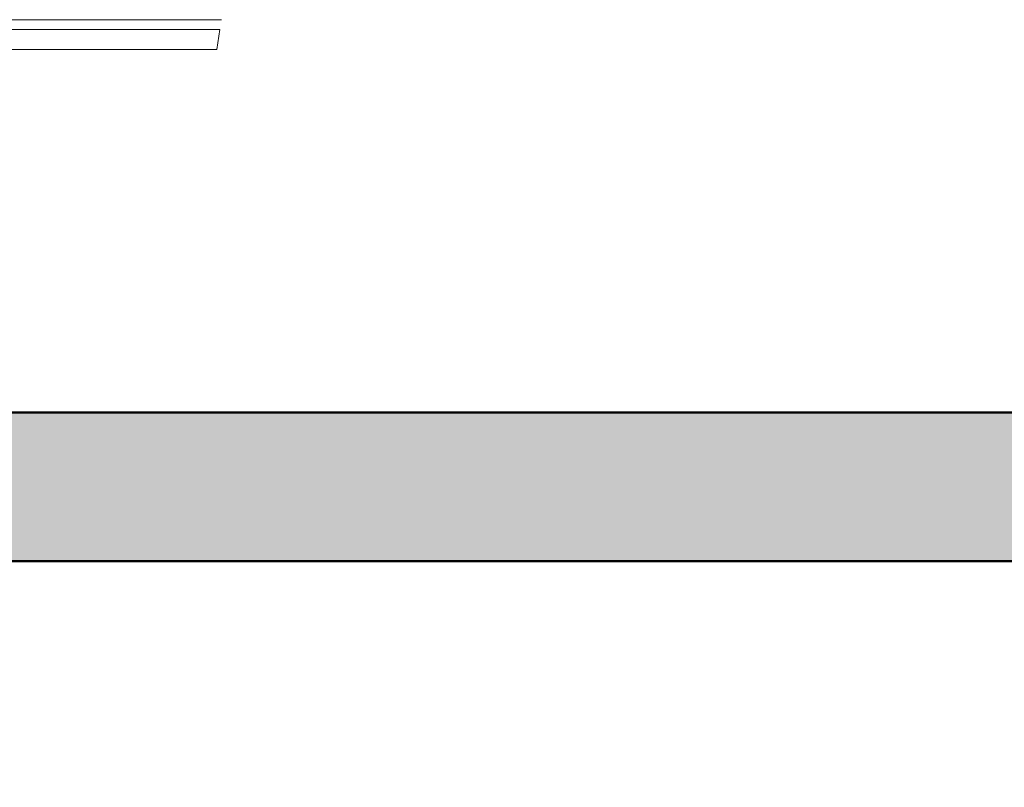
# Model space of a CAD drawing. Units: inches. Extents: x 2419 to 2878, y 1068 to 1713.
# Tile 5 of 20: x 2541 to 2574, y 1286 to 1312. Entities that reach past the tile are written whole.
import ezdxf

# ---------------------------------------------------------------- set-up
doc = ezdxf.new("R2010")
doc.units = ezdxf.units.IN
for name, color, linetype, lineweight in [('A-ANNO-DIMS', 2, 'Continuous', 18), ('A-FLOR-PRKG-PATT', 1, 'Continuous', 13), ('A-FURN', 8, 'Continuous', 18), ('A-WALL', 7, 'Continuous', 50)]:
    doc.layers.add(name, color=color, linetype=linetype, lineweight=lineweight)
doc.layers.add('A-WALL-PATT', color=18, linetype='Continuous', lineweight=13, true_color=0x000000)
doc.styles.get("Standard").update_dxf_attribs({"font": 'arial.ttf'})
doc.dimstyles.new('ISO-25', dxfattribs={"dimtxt": 12.5, "dimasz": 2.5, "dimexe": 1.25, "dimexo": 0.625, "dimtad": 1, "dimdec": 0, "dimlunit": 4, "dimtxsty": 'Standard', "dimblk": 'ARCHTICK', "dimcen": 2.5, "dimse1": 1, "dimse2": 1, "dimclrd": 4, "dimadec": 0, "dimazin": 0, "dimtfac": 1, "dimtdec": 0, "dimtmove": 0, "dimatfit": 3, "dimfxl": 1, "dimarcsym": 0})

# ---------------------------------------------------------------- blocks, each defined once
blk = doc.blocks.new('Dining Set - 36 x 72 in.')
for p, q in [((5.7696, -26), (22.2392, -26)), ((22.1584, -26.5), (5.8466, -26.5)), ((22.1563, -26.49967), (22, -27.5)), ((6, -27.5), (22, -27.5))]:
    blk.add_line(p, q)
blk = doc.blocks.new('_ArchTick')
at = {"color": 0, "linetype": 'ByBlock', "const_width": 0.15}
blk.add_lwpolyline([(-0.5, -0.5), (0.5, 0.5)], dxfattribs=at)
blk = doc.blocks.new('*D43')
at = {"layer": 'A-ANNO-DIMS', "color": 4, "lineweight": -2, "transparency": 16777216}
blk.add_line((2480.514, 1079.925), (2557.299, 1079.925), dxfattribs=at)
at = {"layer": 'Defpoints', "color": 0, "transparency": 16777216}
for p in [(2480.514, 1408.813), (2557.299, 1408.813), (2557.299, 1079.925)]:
    blk.add_point(p, dxfattribs=at)
at = {"layer": 'A-ANNO-DIMS', "color": 4, "lineweight": -2, "transparency": 16777216, "xscale": 2.5, "yscale": 2.5, "zscale": 2.5, "rotation": 180}
blk.add_blockref('_ArchTick', (2480.514, 1079.925), dxfattribs=at)
at = {"layer": 'A-ANNO-DIMS', "color": 4, "lineweight": -2, "transparency": 16777216, "xscale": 2.5, "yscale": 2.5, "zscale": 2.5}
blk.add_blockref('_ArchTick', (2557.299, 1079.925), dxfattribs=at)
at = {"layer": 'A-ANNO-DIMS', "color": 0, "transparency": 16777216, "insert": (2518.907, 1086.932), "char_height": 12.5, "attachment_point": 5}
blk.add_mtext('6\'-5"', dxfattribs=at)
blk = doc.blocks.new('*D44')
at = {"layer": 'A-ANNO-DIMS', "color": 4, "lineweight": -2, "transparency": 16777216}
for p, q in [((2557.299, 1079.925), (2585.818, 1079.925)), ((2585.818, 1079.925), (2652.136, 1079.925))]:
    blk.add_line(p, q, dxfattribs=at)
at = {"layer": 'Defpoints', "color": 0, "transparency": 16777216}
for p in [(2557.299, 1408.813), (2585.818, 1408.813), (2585.818, 1079.925)]:
    blk.add_point(p, dxfattribs=at)
at = {"layer": 'A-ANNO-DIMS', "color": 4, "lineweight": -2, "transparency": 16777216, "xscale": 2.5, "yscale": 2.5, "zscale": 2.5, "rotation": 180}
blk.add_blockref('_ArchTick', (2557.299, 1079.925), dxfattribs=at)
at = {"layer": 'A-ANNO-DIMS', "color": 4, "lineweight": -2, "transparency": 16777216, "xscale": 2.5, "yscale": 2.5, "zscale": 2.5}
blk.add_blockref('_ArchTick', (2585.818, 1079.925), dxfattribs=at)
at = {"layer": 'A-ANNO-DIMS', "color": 0, "transparency": 16777216, "insert": (2620.227, 1087.013), "char_height": 12.5, "attachment_point": 5}
blk.add_mtext('2\'-4 1/2"', dxfattribs=at)
blk = doc.blocks.new('*D47')
at = {"layer": 'A-ANNO-DIMS', "color": 4, "lineweight": -2, "transparency": 16777216}
for p, q in [((2444.314, 1376.561), (2444.314, 1357.976)), ((2444.314, 1357.976), (2444.314, 1293.048))]:
    blk.add_line(p, q, dxfattribs=at)
at = {"layer": 'Defpoints', "color": 0, "transparency": 16777216}
for p in [(2632.514, 1376.561), (2444.314, 1357.976), (2632.514, 1357.976)]:
    blk.add_point(p, dxfattribs=at)
at = {"layer": 'A-ANNO-DIMS', "color": 4, "lineweight": -2, "transparency": 16777216, "xscale": 2.5, "yscale": 2.5, "zscale": 2.5}
for p, rotation in [((2444.314, 1376.561), 90), ((2444.314, 1357.976), 270)]:
    blk.add_blockref('_ArchTick', p, dxfattribs=dict(at, rotation=rotation))
at = {"layer": 'A-ANNO-DIMS', "color": 0, "transparency": 16777216, "insert": (2437.226, 1324.262), "char_height": 12.5, "attachment_point": 5, "rotation": 90}
blk.add_mtext('1\'-6 1/2"', dxfattribs=at)
blk = doc.blocks.new('*D56')
at = {"layer": 'A-ANNO-DIMS', "color": 4, "lineweight": -2, "transparency": 16777216}
for p, q in [((2480.514, 1079.925), (2503.967, 1079.925)), ((2503.967, 1079.925), (2578.607, 1079.925))]:
    blk.add_line(p, q, dxfattribs=at)
at = {"layer": 'Defpoints', "color": 0, "transparency": 16777216}
for p in [(2480.514, 1507.813), (2503.967, 1494.852), (2503.967, 1079.925)]:
    blk.add_point(p, dxfattribs=at)
at = {"layer": 'A-ANNO-DIMS', "color": 4, "lineweight": -2, "transparency": 16777216, "xscale": 2.5, "yscale": 2.5, "zscale": 2.5, "rotation": 180}
blk.add_blockref('_ArchTick', (2480.514, 1079.925), dxfattribs=at)
at = {"layer": 'A-ANNO-DIMS', "color": 4, "lineweight": -2, "transparency": 16777216, "xscale": 2.5, "yscale": 2.5, "zscale": 2.5}
blk.add_blockref('_ArchTick', (2503.967, 1079.925), dxfattribs=at)
at = {"layer": 'A-ANNO-DIMS', "color": 0, "transparency": 16777216, "insert": (2542.537, 1087.013), "char_height": 12.5, "attachment_point": 5}
blk.add_mtext('1\'-11 1/2"', dxfattribs=at)
blk = doc.blocks.new('*D59')
at = {"layer": 'A-ANNO-DIMS', "color": 4, "lineweight": -2, "transparency": 16777216}
blk.add_line((2480.514, 1079.925), (2589.514, 1079.925), dxfattribs=at)
at = {"layer": 'Defpoints', "color": 0, "transparency": 16777216}
for p in [(2480.514, 1414.813), (2589.514, 1414.813), (2589.514, 1079.925)]:
    blk.add_point(p, dxfattribs=at)
at = {"layer": 'A-ANNO-DIMS', "color": 4, "lineweight": -2, "transparency": 16777216, "xscale": 2.5, "yscale": 2.5, "zscale": 2.5, "rotation": 180}
blk.add_blockref('_ArchTick', (2480.514, 1079.925), dxfattribs=at)
at = {"layer": 'A-ANNO-DIMS', "color": 4, "lineweight": -2, "transparency": 16777216, "xscale": 2.5, "yscale": 2.5, "zscale": 2.5}
blk.add_blockref('_ArchTick', (2589.514, 1079.925), dxfattribs=at)
at = {"layer": 'A-ANNO-DIMS', "color": 0, "transparency": 16777216, "insert": (2535.014, 1086.932), "char_height": 12.5, "attachment_point": 5}
blk.add_mtext('9\'-1"', dxfattribs=at)

msp = doc.modelspace()

# ---------------------------------------------------------------- hatches: boundary and pattern name
at = {"layer": 'A-FLOR-PRKG-PATT'}
h = msp.add_hatch(color=256, dxfattribs=at)
h.dxf.hatch_style = 1
edge = h.paths.add_edge_path()
edge.add_ellipse((2561.374, 1279.453), major_axis=(3.988, 0), ratio=0.842304, start_angle=0.6466, end_angle=90)
edge.add_line((2561.374, 1282.813), (2511.571, 1282.813))
edge.add_ellipse((2511.571, 1279.453), major_axis=(3.988, 0), ratio=0.842304, start_angle=90, end_angle=179.3534)
edge.add_ellipse((10560.892, 1188.617), major_axis=(-8054.031, 0), ratio=0.84230387, start_angle=-0.6465541, end_angle=-0.6282372)
edge.add_ellipse((2509.23, 1276.906), major_axis=(1.687, 0), ratio=0.842304, start_angle=179.3718, end_angle=248.4648)
edge.add_ellipse((10560.329, 1188.617), major_axis=(8052.293, 0), ratio=0.84230387, start_angle=179.3534459, end_angle=179.3813568, ccw=False)
edge.add_ellipse((2511.008, 1279.453), major_axis=(2.25, 0), ratio=0.842304, start_angle=90, end_angle=179.3534, ccw=False)
edge.add_line((2511.008, 1281.348), (2561.936, 1281.348))
edge.add_ellipse((2561.936, 1279.453), major_axis=(-2.25, 0), ratio=0.842304, start_angle=180.6466, end_angle=270, ccw=False)
edge.add_ellipse((-5487.385, 1188.617), major_axis=(8052.293, 0), ratio=0.84230387, start_angle=0.5282715, end_angle=0.6465541, ccw=False)
edge.add_ellipse((2563.715, 1276.906), major_axis=(-1.687, 0), ratio=0.842304, start_angle=111.5352, end_angle=180.6282)
edge.add_ellipse((-5487.947, 1188.617), major_axis=(-8054.031, 0), ratio=0.84230387, start_angle=180.6282372, end_angle=180.6465541)
edge = h.paths.add_edge_path()
edge.add_ellipse((2564.908, 1261.91), major_axis=(-1.125, 0), ratio=0.842304, start_angle=180, end_angle=270)
edge.add_line((2564.908, 1262.857), (2564.426, 1262.857))
edge.add_ellipse((-5487.385, 1188.617), major_axis=(8052.293, 0), ratio=0.84230387, start_angle=0.3838668, end_angle=0.5282715, ccw=False)
edge.add_line((2564.654, 1242.564), (2564.908, 1242.564))
edge.add_ellipse((2564.908, 1243.512), major_axis=(-1.125, 0), ratio=0.842304, start_angle=90, end_angle=180)
edge.add_line((2566.033, 1243.512), (2566.033, 1261.91))
edge = h.paths.add_edge_path()
edge.add_ellipse((2564.908, 1174.989), major_axis=(1.125, 0), ratio=0.842304, start_angle=0, end_angle=90)
edge.add_line((2564.908, 1175.936), (2564.894, 1175.936))
edge.add_ellipse((-5487.385, 1188.617), major_axis=(8052.293, 0), ratio=0.84230387, start_angle=-0.1349866, end_angle=-0.0902291, ccw=False)
edge.add_ellipse((2163.343, 1170.913), major_axis=(401.537, 0), ratio=0.8423039, start_angle=-2.17995, end_angle=-0.13561, ccw=False)
edge.add_line((2564.47, 1155.643), (2564.908, 1155.643))
edge.add_ellipse((2564.908, 1156.591), major_axis=(-1.125, 0), ratio=0.842304, start_angle=90, end_angle=180)
edge.add_line((2566.033, 1156.591), (2566.033, 1174.989))
h.paths.add_polyline_path([(2574.476, 1207.448), (2633.94, 1207.448), (2633.94, 1217.366), (2574.476, 1217.366)], flags=9)
h.paths.add_polyline_path([(2574.454, 1217.828), (2610.472, 1217.828), (2610.472, 1227.879), (2574.454, 1227.879)], flags=9)
h.paths.add_polyline_path([(2672.426, 1304.02), (2718.617, 1304.02), (2718.617, 1313.939), (2672.426, 1313.939)], flags=9)
h.paths.add_polyline_path([(2672.404, 1314.4), (2750.128, 1314.4), (2750.128, 1324.451), (2672.404, 1324.451)], flags=9)
h.paths.add_polyline_path([(2500.432, 1374.444), (2544.803, 1374.444), (2544.803, 1384.362), (2500.432, 1384.362)], flags=9)
h.paths.add_polyline_path([(2500.41, 1384.824), (2566.075, 1384.824), (2566.075, 1394.875), (2500.41, 1394.875)], flags=9)
h.paths.add_polyline_path([(2738.933, 1376.749), (2778.273, 1376.749), (2778.273, 1386.667), (2738.933, 1386.667)], flags=9)
h.paths.add_polyline_path([(2659.12, 1357.8), (2703.492, 1357.8), (2703.492, 1367.718), (2659.12, 1367.718)], flags=9)
h.paths.add_polyline_path([(2659.098, 1368.18), (2694.114, 1368.18), (2694.114, 1378.23), (2659.098, 1378.23)], flags=9)
h.paths.add_polyline_path([(2730.123, 1466.067), (2769.463, 1466.067), (2769.463, 1475.986), (2730.123, 1475.986)], flags=9)
h.paths.add_polyline_path([(2730.101, 1476.447), (2765.117, 1476.447), (2765.117, 1486.498), (2730.101, 1486.498)], flags=9)
h.paths.add_polyline_path([(2730.382, 1518.647), (2761.48, 1518.647), (2761.48, 1528.566), (2730.382, 1528.566)], flags=9)
h.paths.add_polyline_path([(2730.361, 1529.028), (2780.958, 1529.028), (2780.958, 1539.072), (2730.361, 1539.072)], flags=9)
h.paths.add_polyline_path([(2629.32, 1455.189), (2688.784, 1455.189), (2688.784, 1465.107), (2629.32, 1465.107)], flags=9)
h.paths.add_polyline_path([(2629.298, 1465.569), (2681.902, 1465.569), (2681.902, 1475.62), (2629.298, 1475.62)], flags=9)
h.paths.add_polyline_path([(2513.229, 1456.484), (2562.631, 1456.484), (2562.631, 1466.402), (2513.229, 1466.402)], flags=9)
h.paths.add_polyline_path([(2513.208, 1466.865), (2556.26, 1466.865), (2556.26, 1476.909), (2513.208, 1476.909)], flags=9)
h.paths.add_polyline_path([(2488.87, 1521.538), (2519.968, 1521.538), (2519.968, 1531.456), (2488.87, 1531.456)], flags=9)
h.paths.add_polyline_path([(2536.549, 1543.507), (2580.923, 1543.507), (2580.923, 1553.432), (2536.549, 1553.432)], flags=9)
h.paths.add_polyline_path([(2536.557, 1553.921), (2573.525, 1553.921), (2573.525, 1563.8), (2536.557, 1563.8)], flags=9)
at = {"layer": 'A-WALL-PATT'}
h = msp.add_hatch(color=256, dxfattribs=at)
h.dxf.hatch_style = 1
h.paths.add_polyline_path([(2780.514, 1577.813), (2471.514, 1577.813), (2471.514, 1121.813), (2780.514, 1121.813)])
h.paths.add_polyline_path([(2480.514, 1568.813), (2771.514, 1568.813), (2771.514, 1130.813), (2480.514, 1130.813)], flags=16)
h.paths.add_polyline_path([(2528.514, 1568.813), (2528.514, 1512.813), (2594.514, 1512.813), (2594.514, 1414.813), (2596.568, 1414.813), (2596.568, 1441.609), (2597.816, 1441.609), (2597.816, 1441.582, -0.384016), (2625.035, 1414.813), (2725.514, 1414.813), (2725.514, 1567.545), (2728.302, 1567.545), (2746.887, 1567.545), (2746.887, 1566.732), (2746.87, 1566.732, -0.367216), (2730.514, 1549.092), (2730.514, 1512.813), (2750.853, 1512.813), (2750.853, 1510.025, -0.401453), (2733.081, 1491.458), (2733.081, 1491.44), (2732.268, 1491.44), (2732.268, 1507.813), (2730.514, 1507.813), (2730.514, 1408.813), (2736.514, 1408.813), (2736.514, 1349.813), (2632.514, 1349.813), (2632.514, 1408.813), (2528.514, 1408.813), (2528.514, 1414.813), (2503.967, 1414.813), (2503.967, 1494.852), (2558.379, 1494.852), (2558.379, 1507.813), (2529.965, 1507.813, -0.414214), (2530.821, 1506.957), (2530.821, 1497.257, -0.414214), (2529.965, 1496.401), (2514.559, 1496.401, -0.414214), (2513.703, 1497.257), (2513.703, 1506.957, -0.414214), (2514.559, 1507.813), (2528.514, 1507.813), (2528.514, 1512.813), (2480.514, 1512.813)], flags=0)
h.paths.add_polyline_path([(2516.262, 1507.813), (2528.262, 1507.813), (2528.262, 1505.813), (2523.417, 1505.813), (2524.074, 1504.675), (2529.394, 1504.675, -0.414214), (2529.965, 1504.104), (2529.965, 1497.828, -0.414214), (2529.394, 1497.257), (2515.13, 1497.257, -0.414214), (2514.559, 1497.828), (2514.559, 1504.104, -0.414214), (2515.13, 1504.675), (2520.689, 1504.675), (2521.342, 1505.813), (2516.262, 1505.813)], flags=0)
h.paths.add_polyline_path([(2522.016, 1505.531), (2522.817, 1507.318, -0.65506), (2522.254, 1506.063), (2522.195, 1505.93), (2522.425, 1505.531)], flags=0)
h.paths.add_polyline_path([(2522.833, 1500.966, -1), (2521.691, 1500.966, -1)], flags=0)
h.paths.add_polyline_path([(2522.547, 1500.966, -1), (2521.977, 1500.966, -1)], flags=0)
h.paths.add_polyline_path([(2482.005, 1470.633), (2499.894, 1470.633), (2499.894, 1448.272), (2482.005, 1448.272), (2482.005, 1452.744), (2481.26, 1452.744), (2481.26, 1449.763), (2480.514, 1449.763), (2480.514, 1469.142), (2481.26, 1469.142), (2481.26, 1466.16), (2482.005, 1466.16)], flags=0)
h.paths.add_polyline_path([(2488.713, 1466.16, -1), (2484.241, 1466.16, -1)], flags=0)
h.paths.add_polyline_path([(2496.167, 1466.16, -1), (2490.204, 1466.16, -1)], flags=0)
h.paths.add_polyline_path([(2487.968, 1466.16, -1), (2484.987, 1466.16, -1)], flags=0)
h.paths.add_polyline_path([(2495.422, 1466.16, -1), (2490.949, 1466.16, -1)], flags=0)
h.paths.add_polyline_path([(2487.223, 1466.16, -1), (2485.732, 1466.16, -1)], flags=0)
h.paths.add_polyline_path([(2494.676, 1466.16, -1), (2491.695, 1466.16, -1)], flags=0)
h.paths.add_polyline_path([(2499.108, 1468.005, -1), (2497.977, 1468.005, -1)], flags=0)
h.paths.add_polyline_path([(2493.931, 1466.16, -1), (2492.44, 1466.16, -1)], flags=0)
h.paths.add_polyline_path([(2499.372, 1463.71, -1), (2498.166, 1463.71, -1)], flags=0)
h.paths.add_polyline_path([(2484.241, 1461.688), (2496.167, 1461.688), (2496.167, 1457.216), (2484.241, 1457.216)], flags=0)
h.paths.add_polyline_path([(2484.987, 1460.943), (2495.422, 1460.943), (2495.422, 1457.961), (2484.987, 1457.961)], flags=0)
h.paths.add_polyline_path([(2586.88, 1510.025), (2587.693, 1510.025), (2587.693, 1491.44), (2586.88, 1491.44)], flags=0)
h.paths.add_polyline_path([(2499.259, 1459.415, -1), (2498.203, 1459.415, -1)], flags=0)
h.paths.add_polyline_path([(2489.459, 1452.744, -1), (2483.496, 1452.744, -1)], flags=0)
h.paths.add_polyline_path([(2557.299, 1408.813), (2557.299, 1413.091, -0.401453), (2584.57, 1441.582), (2584.57, 1441.609), (2585.818, 1441.609), (2585.818, 1413.091), (2585.818, 1408.813)], flags=0)
h.paths.add_polyline_path([(2488.713, 1452.744, -1), (2484.241, 1452.744, -1)], flags=0)
h.paths.add_polyline_path([(2495.422, 1452.744, -1), (2490.949, 1452.744, -1)], flags=0)
h.paths.add_polyline_path([(2487.968, 1452.744, -1), (2484.987, 1452.744, -1)], flags=0)
h.paths.add_polyline_path([(2494.676, 1452.744, -1), (2491.695, 1452.744, -1)], flags=0)
h.paths.add_polyline_path([(2487.223, 1452.744, -1), (2485.732, 1452.744, -1)], flags=0)
h.paths.add_polyline_path([(2499.183, 1454.442, -1), (2497.902, 1454.442, -1)], flags=0)
h.paths.add_polyline_path([(2493.931, 1452.744, -1), (2492.44, 1452.744, -1)], flags=0)
h.paths.add_polyline_path([(2499.296, 1450.637, -1), (2497.789, 1450.637, -1)], flags=0)
h.paths.add_polyline_path([(2619.129, 1558.889, -1), (2605.129, 1558.889, -1)], flags=0)
h.paths.add_polyline_path([(2609.129, 1558.889), (2612.129, 1561.889), (2615.129, 1558.889), (2612.129, 1555.889)], flags=0)
h.paths.add_polyline_path([(2611.129, 1558.889, -1), (2613.129, 1558.889, -1)], flags=0)
h.paths.add_polyline_path([(2633.679, 1568.813), (2693.679, 1568.813), (2693.679, 1488.813), (2633.679, 1488.813)], flags=0)
h.paths.add_polyline_path([(2641.679, 1554.413), (2641.679, 1567.613), (2662.479, 1567.613), (2662.479, 1554.413), (2664.879, 1554.413), (2664.879, 1567.613), (2685.679, 1567.613), (2685.679, 1552.413), (2680.479, 1552.413), (2693.679, 1539.213), (2678.479, 1539.213), (2678.479, 1554.413)], flags=0)
h.paths.add_polyline_path([(2637.514, 1408.813), (2731.514, 1408.813), (2731.514, 1354.813), (2637.514, 1354.813), (2637.514, 1357.976), (2635.302, 1357.976), (2635.302, 1358.789), (2637.514, 1358.789)], flags=0)
h.paths.add_polyline_path([(2717.171, 1559.643, -1), (2703.171, 1559.643, -1)], flags=0)
h.paths.add_polyline_path([(2707.171, 1559.643), (2710.171, 1562.643), (2713.171, 1559.643), (2710.171, 1556.643)], flags=0)
h.paths.add_polyline_path([(2709.171, 1559.643, -1), (2711.171, 1559.643, -1)], flags=0)
h.paths.add_polyline_path([(2685.378, 1408.813), (2706.378, 1408.813), (2706.378, 1400.813), (2699.878, 1400.813), (2701.878, 1394.813, -0.501323), (2696.923, 1375.952, -0.132891), (2694.834, 1375.952, -0.501317), (2689.878, 1394.813), (2691.878, 1400.813), (2688.878, 1400.813), (2688.878, 1399.313), (2685.878, 1399.313), (2685.878, 1400.313), (2687.878, 1400.313), (2687.878, 1400.813), (2685.378, 1400.813)], flags=0)
h.paths.add_polyline_path([(2687.378, 1407.813), (2704.378, 1407.813, -0.5), (2705.378, 1406.813), (2705.378, 1402.813, -0.5), (2704.378, 1401.813), (2687.378, 1401.813, -0.5), (2686.378, 1402.813), (2686.378, 1406.813, -0.5)], flags=0)
h.paths.add_polyline_path([(2639.514, 1205.813), (2634.514, 1205.813), (2634.514, 1293.813), (2637.514, 1293.813), (2639.514, 1293.813)], flags=0)
h.paths.add_polyline_path([(2691.878, 1394.813), (2699.878, 1394.813, -0.48008), (2697.522, 1377.29, -0.215004), (2694.234, 1377.29, -0.48008)], flags=0)
h.paths.add_polyline_path([(2757.514, 1453.891), (2763.514, 1451.891), (2763.514, 1454.891), (2762.014, 1454.891), (2762.014, 1457.891), (2763.014, 1457.891), (2763.014, 1455.891), (2763.514, 1455.891), (2763.514, 1458.391), (2771.514, 1458.391), (2771.514, 1437.391), (2763.514, 1437.391), (2763.514, 1443.891), (2757.515, 1441.891, -0.501323), (2738.653, 1446.847, -0.132891), (2738.653, 1448.936, -0.501317)], flags=0)
h.paths.add_polyline_path([(2739.991, 1449.535, -0.48008), (2757.514, 1451.891), (2757.514, 1443.891, -0.48008), (2739.991, 1446.247, -0.215004)], flags=0)
h.paths.add_polyline_path([(2765.514, 1457.391), (2769.514, 1457.391, -0.5), (2770.514, 1456.391), (2770.514, 1439.391, -0.5), (2769.514, 1438.391), (2765.514, 1438.391, -0.5), (2764.514, 1439.391), (2764.514, 1456.391, -0.5)], flags=0)
h = msp.add_hatch(color=256, dxfattribs=at)
h.dxf.hatch_style = 1
h.paths.add_polyline_path([(2771.514, 1354.813), (2736.514, 1354.813), (2736.514, 1408.813), (2771.514, 1408.813), (2771.514, 1414.813), (2625.035, 1414.813, -0.015108), (2625.087, 1413.091), (2625.087, 1408.813), (2632.514, 1408.813), (2632.514, 1376.561), (2635.302, 1376.561, -0.029838), (2637.514, 1376.429), (2637.514, 1408.813), (2731.514, 1408.813), (2731.514, 1354.813), (2637.514, 1354.813), (2637.514, 1357.976), (2635.302, 1357.976), (2632.514, 1357.976), (2632.514, 1349.813), (2771.514, 1349.813)])
h.paths.add_polyline_path([(2639.514, 1298.813), (2637.514, 1298.813), (2480.514, 1298.813), (2480.514, 1293.813), (2637.514, 1293.813), (2639.514, 1293.813)])
h.paths.add_polyline_path([(2639.514, 1293.813), (2637.514, 1293.813), (2634.514, 1293.813), (2634.514, 1244.653), (2638.792, 1244.653, -0.006332), (2639.514, 1244.644)])
h.paths.add_polyline_path([(2639.514, 1205.813), (2771.514, 1205.813), (2771.514, 1210.813), (2639.514, 1210.813), (2639.514, 1216.134), (2638.792, 1216.134), (2634.514, 1216.134), (2634.514, 1130.813), (2639.514, 1130.813)])
h.paths.add_polyline_path([(2596.568, 1413.091), (2596.568, 1414.813), (2585.818, 1414.813), (2585.818, 1413.091), (2585.818, 1408.813), (2596.568, 1408.813)])
h.paths.add_polyline_path([(2557.299, 1413.091, -0.015108), (2557.351, 1414.813), (2480.514, 1414.813), (2480.514, 1408.813), (2557.299, 1408.813)])
h.paths.add_polyline_path([(2574.476, 1207.448), (2633.94, 1207.448), (2633.94, 1217.366), (2574.476, 1217.366)], flags=9)
h.paths.add_polyline_path([(2574.454, 1217.828), (2610.472, 1217.828), (2610.472, 1227.879), (2574.454, 1227.879)], flags=9)
h.paths.add_polyline_path([(2672.426, 1304.02), (2718.617, 1304.02), (2718.617, 1313.939), (2672.426, 1313.939)], flags=9)
h.paths.add_polyline_path([(2672.404, 1314.4), (2750.128, 1314.4), (2750.128, 1324.451), (2672.404, 1324.451)], flags=9)
h.paths.add_polyline_path([(2500.432, 1374.444), (2544.803, 1374.444), (2544.803, 1384.362), (2500.432, 1384.362)], flags=9)
h.paths.add_polyline_path([(2500.41, 1384.824), (2566.075, 1384.824), (2566.075, 1394.875), (2500.41, 1394.875)], flags=9)
h.paths.add_polyline_path([(2738.933, 1376.749), (2778.273, 1376.749), (2778.273, 1386.667), (2738.933, 1386.667)], flags=9)
h.paths.add_polyline_path([(2659.12, 1357.8), (2703.492, 1357.8), (2703.492, 1367.718), (2659.12, 1367.718)], flags=25)
h.paths.add_polyline_path([(2659.098, 1368.18), (2694.114, 1368.18), (2694.114, 1378.23), (2659.098, 1378.23)], flags=25)
h.paths.add_polyline_path([(2730.123, 1466.067), (2769.463, 1466.067), (2769.463, 1475.986), (2730.123, 1475.986)], flags=9)
h.paths.add_polyline_path([(2730.101, 1476.447), (2765.117, 1476.447), (2765.117, 1486.498), (2730.101, 1486.498)], flags=9)
h.paths.add_polyline_path([(2730.382, 1518.647), (2761.48, 1518.647), (2761.48, 1528.566), (2730.382, 1528.566)], flags=9)
h.paths.add_polyline_path([(2730.361, 1529.028), (2780.958, 1529.028), (2780.958, 1539.072), (2730.361, 1539.072)], flags=9)
h.paths.add_polyline_path([(2629.32, 1455.189), (2688.784, 1455.189), (2688.784, 1465.107), (2629.32, 1465.107)], flags=9)
h.paths.add_polyline_path([(2629.298, 1465.569), (2681.902, 1465.569), (2681.902, 1475.62), (2629.298, 1475.62)], flags=9)
h.paths.add_polyline_path([(2513.229, 1456.484), (2562.631, 1456.484), (2562.631, 1466.402), (2513.229, 1466.402)], flags=9)
h.paths.add_polyline_path([(2513.208, 1466.865), (2556.26, 1466.865), (2556.26, 1476.909), (2513.208, 1476.909)], flags=9)
h.paths.add_polyline_path([(2488.87, 1521.538), (2519.968, 1521.538), (2519.968, 1531.456), (2488.87, 1531.456)], flags=9)
h.paths.add_polyline_path([(2536.549, 1543.507), (2580.923, 1543.507), (2580.923, 1553.432), (2536.549, 1553.432)], flags=9)
h.paths.add_polyline_path([(2536.557, 1553.921), (2573.525, 1553.921), (2573.525, 1563.8), (2536.557, 1563.8)], flags=9)

# ---------------------------------------------------------------- linework, layer by layer
at = {"layer": 'A-WALL'}
for p, q in [((2480.514, 1298.813), (2637.514, 1298.813)), ((2480.514, 1293.813), (2637.514, 1293.813))]:
    msp.add_line(p, q, dxfattribs=at)

# ---------------------------------------------------------------- block references
at = {"layer": 'A-FURN', "xscale": 0.6669202688727635, "yscale": 0.6669202688727635, "zscale": 0.6669202688727635}
msp.add_blockref('Dining Set - 36 x 72 in.', (2533.113, 1329.346), dxfattribs=at)

# ---------------------------------------------------------------- dimensions: what is measured, and where the dimension line sits
at = {"layer": 'A-ANNO-DIMS'}
for base, p1, p2, picture, middle in [((2503.967, 1079.925), (2480.514, 1507.813), (2503.967, 1494.852), '*D56', (2542.537, 1087.013)), ((2589.514, 1079.925), (2480.514, 1414.813), (2589.514, 1414.813), '*D59', (2535.014, 1086.932)), ((2557.299, 1079.925), (2480.514, 1408.813), (2557.299, 1408.813), '*D43', (2518.907, 1086.932)), ((2585.818, 1079.925), (2557.299, 1408.813), (2585.818, 1408.813), '*D44', (2620.227, 1087.013))]:
    dim = msp.add_linear_dim(base=base, p1=p1, p2=p2, dimstyle='ISO-25', override={"dimdec": 1, "dimlfac": 1, "dimrnd": 0, "dimzin": 1, "dimdsep": 46, "dimlunit": 4, "dimfrac": 2}, dxfattribs=at)
    dim.commit()
    dim.dimension.update_dxf_attribs({"geometry": picture, "text_midpoint": middle})
dim = msp.add_linear_dim(base=(2444.314, 1357.976), p1=(2632.514, 1376.561), p2=(2632.514, 1357.976), angle=90, dimstyle='ISO-25', override={"dimdec": 1, "dimlfac": 1, "dimrnd": 0, "dimzin": 1, "dimdsep": 46, "dimlunit": 4, "dimfrac": 2}, dxfattribs=at)
dim.commit()
dim.dimension.update_dxf_attribs({"geometry": '*D47', "text_midpoint": (2437.226, 1324.262)})

doc.saveas('drawing.dxf')
